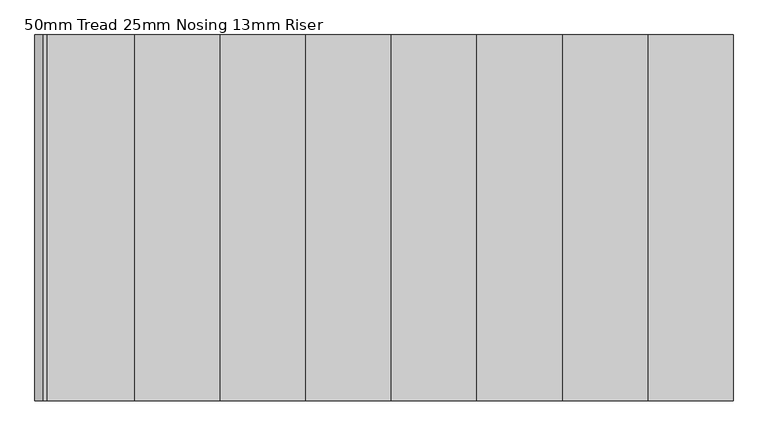
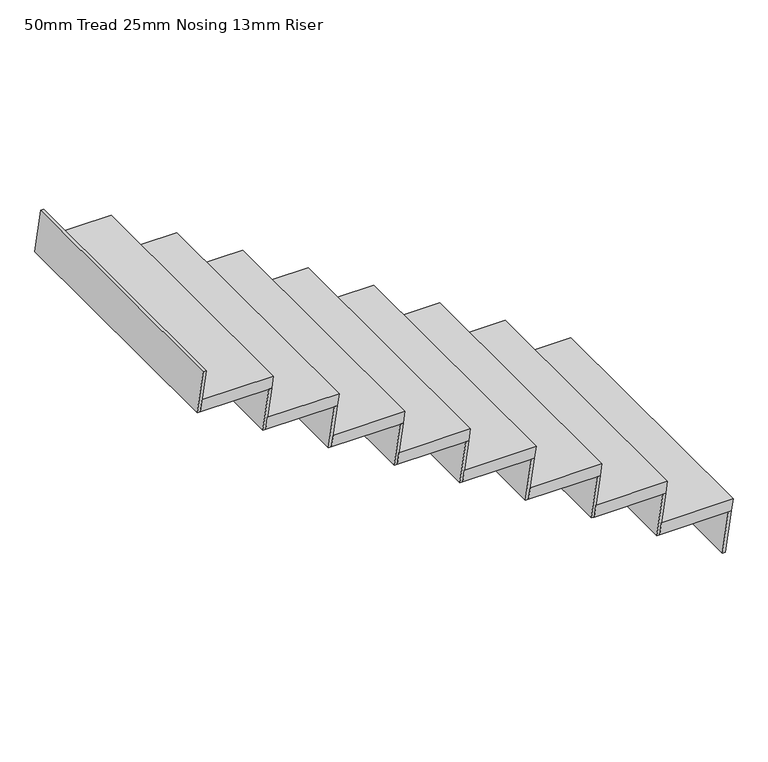
"""IFC4 building model written with IfcOpenShell, lengths in millimetres: stair flight geometry, 50mm Tread 25mm Nosing 13mm Riser."""

from ifc_helpers import new_model, si_unit, frame, origin, place, context, project, spatial, polyline, outline, extrude, source, transform, mapped, element, save


def stair_flight_50mm_tread_25mm_nosing_13mm_riser_1a1c1790(model_context):
    return source(origin(), model_context, "Body", "SweptSolid", [
        extrude(outline(polyline([(1391.3043478, 692.2052675), (1391.3043478, 392.2052675), (1341.3043478, 385.0177675), (1341.3043478, 685.0177675), (1391.3043478, 692.2052675)])), frame((0.0, 4668.9227481, 0.0), z_axis=(0.0, 1.0, 0.0), x_axis=(0.0, 0.0, 1.0)), (0.0, 0.0, 1.0), 1176.2290046),
        extrude(outline(polyline([(1341.3043478, 685.0177675), (1341.3043478, 672.3892775), (1167.3913043, 647.3892775), (1167.3913043, 660.0177675), (1341.3043478, 685.0177675)])), frame((0.0, 4668.9227481, 0.0), z_axis=(0.0, 1.0, 0.0), x_axis=(0.0, 0.0, 1.0)), (0.0, 0.0, 1.0), 1176.2290046),
        extrude(outline(polyline([(1515.2173913, 410.0177675), (1515.2173913, 397.3892775), (1341.3043478, 372.3892775), (1341.3043478, 385.0177675), (1515.2173913, 410.0177675)])), frame((0.0, 4668.9227481, 0.0), z_axis=(0.0, 1.0, 0.0), x_axis=(0.0, 0.0, 1.0)), (0.0, 0.0, 1.0), 1176.2290046),
        extrude(outline(polyline([(1565.2173913, 417.2052675), (1565.2173913, 117.2052675), (1515.2173913, 110.0177675), (1515.2173913, 410.0177675), (1565.2173913, 417.2052675)])), frame((0.0, 4668.9227481, 0.0), z_axis=(0.0, 1.0, 0.0), x_axis=(0.0, 0.0, 1.0)), (0.0, 0.0, 1.0), 1176.2290046),
        extrude(outline(polyline([(1689.1304348, 135.0177675), (1689.1304348, 122.3892775), (1515.2173913, 97.3892775), (1515.2173913, 110.0177675), (1689.1304348, 135.0177675)])), frame((0.0, 4668.9227481, 0.0), z_axis=(0.0, 1.0, 0.0), x_axis=(0.0, 0.0, 1.0)), (0.0, 0.0, 1.0), 1176.2290046),
        extrude(outline(polyline([(1739.1304348, 142.2052675), (1739.1304348, -157.7947325), (1689.1304348, -164.9822325), (1689.1304348, 135.0177675), (1739.1304348, 142.2052675)])), frame((0.0, 4668.9227481, 0.0), z_axis=(0.0, 1.0, 0.0), x_axis=(0.0, 0.0, 1.0)), (0.0, 0.0, 1.0), 1176.2290046),
        extrude(outline(polyline([(1863.0434783, -139.9822325), (1863.0434783, -152.6107225), (1689.1304348, -177.6107225), (1689.1304348, -164.9822325), (1863.0434783, -139.9822325)])), frame((0.0, 4668.9227481, 0.0), z_axis=(0.0, 1.0, 0.0), x_axis=(0.0, 0.0, 1.0)), (0.0, 0.0, 1.0), 1176.2290046),
        extrude(outline(polyline([(1913.0434783, -132.7947325), (1913.0434783, -432.7947325), (1863.0434783, -439.9822325), (1863.0434783, -139.9822325), (1913.0434783, -132.7947325)])), frame((0.0, 4668.9227481, 0.0), z_axis=(0.0, 1.0, 0.0), x_axis=(0.0, 0.0, 1.0)), (0.0, 0.0, 1.0), 1176.2290046),
        extrude(outline(polyline([(2036.9565217, -414.9822325), (2036.9565217, -427.6107225), (1863.0434783, -452.6107225), (1863.0434783, -439.9822325), (2036.9565217, -414.9822325)])), frame((0.0, 4668.9227481, 0.0), z_axis=(0.0, 1.0, 0.0), x_axis=(0.0, 0.0, 1.0)), (0.0, 0.0, 1.0), 1176.2290046),
        extrude(outline(polyline([(2086.9565217, -407.7947325), (2086.9565217, -707.7947325), (2036.9565217, -714.9822325), (2036.9565217, -414.9822325), (2086.9565217, -407.7947325)])), frame((0.0, 4668.9227481, 0.0), z_axis=(0.0, 1.0, 0.0), x_axis=(0.0, 0.0, 1.0)), (0.0, 0.0, 1.0), 1176.2290046),
        extrude(outline(polyline([(2210.8695652, -689.9822325), (2210.8695652, -702.6107225), (2036.9565217, -727.6107225), (2036.9565217, -714.9822325), (2210.8695652, -689.9822325)])), frame((0.0, 4668.9227481, 0.0), z_axis=(0.0, 1.0, 0.0), x_axis=(0.0, 0.0, 1.0)), (0.0, 0.0, 1.0), 1176.2290046),
        extrude(outline(polyline([(2260.8695652, -682.7947325), (2260.8695652, -982.7947325), (2210.8695652, -989.9822325), (2210.8695652, -689.9822325), (2260.8695652, -682.7947325)])), frame((0.0, 4668.9227481, 0.0), z_axis=(0.0, 1.0, 0.0), x_axis=(0.0, 0.0, 1.0)), (0.0, 0.0, 1.0), 1176.2290046),
        extrude(outline(polyline([(2384.7826087, -964.9822325), (2384.7826087, -977.6107225), (2210.8695652, -1002.6107225), (2210.8695652, -989.9822325), (2384.7826087, -964.9822325)])), frame((0.0, 4668.9227481, 0.0), z_axis=(0.0, 1.0, 0.0), x_axis=(0.0, 0.0, 1.0)), (0.0, 0.0, 1.0), 1176.2290046),
        extrude(outline(polyline([(2434.7826087, -957.7947325), (2434.7826087, -1257.7947325), (2384.7826087, -1264.9822325), (2384.7826087, -964.9822325), (2434.7826087, -957.7947325)])), frame((0.0, 4668.9227481, 0.0), z_axis=(0.0, 1.0, 0.0), x_axis=(0.0, 0.0, 1.0)), (0.0, 0.0, 1.0), 1176.2290046),
        extrude(outline(polyline([(2558.6956522, -1239.9822325), (2558.6956522, -1252.6107225), (2384.7826087, -1277.6107225), (2384.7826087, -1264.9822325), (2558.6956522, -1239.9822325)])), frame((0.0, 4668.9227481, 0.0), z_axis=(0.0, 1.0, 0.0), x_axis=(0.0, 0.0, 1.0)), (0.0, 0.0, 1.0), 1176.2290046),
        extrude(outline(polyline([(2732.6086957, -1514.9822325), (2732.6086957, -1527.6107225), (2558.6956522, -1552.6107225), (2558.6956522, -1539.9822325), (2732.6086957, -1514.9822325)])), frame((0.0, 4668.9227481, 0.0), z_axis=(0.0, 1.0, 0.0), x_axis=(0.0, 0.0, 1.0)), (0.0, 0.0, 1.0), 1176.2290046),
        extrude(outline(polyline([(2608.6956522, -1232.7947325), (2608.6956522, -1532.7947325), (2558.6956522, -1539.9822325), (2558.6956522, -1239.9822325), (2608.6956522, -1232.7947325)])), frame((0.0, 4668.9227481, 0.0), z_axis=(0.0, 1.0, 0.0), x_axis=(0.0, 0.0, 1.0)), (0.0, 0.0, 1.0), 1176.2290046),
    ])


if __name__ == "__main__":
    model = new_model("IFC4")
    model_context = context("Model", 3, world=origin())
    ifc_project = project(units=[si_unit("LENGTHUNIT", "METRE", prefix="MILLI")], contexts=[model_context])
    site = spatial("IfcSite", under=ifc_project)
    building = spatial("IfcBuilding", under=site)
    placement = place(None, origin())
    stair_flight_50mm_tread_25mm_nosing_13mm_riser_shape = stair_flight_50mm_tread_25mm_nosing_13mm_riser_1a1c1790(model_context)
    element("IfcStairFlight", 1, ObjectType="50mm Tread 25mm Nosing 13mm Riser", at=placement, inside=building, context=model_context, shape_type="MappedRepresentation", body=[
        mapped(stair_flight_50mm_tread_25mm_nosing_13mm_riser_shape, transform((0.0, 0.0, 0.0), x_axis=(1.0, 0.0, 0.0), y_axis=(0.0, 1.0, 0.0), z_axis=(0.0, 0.0, 1.0))),
    ])
    save(model, "model.ifc")
